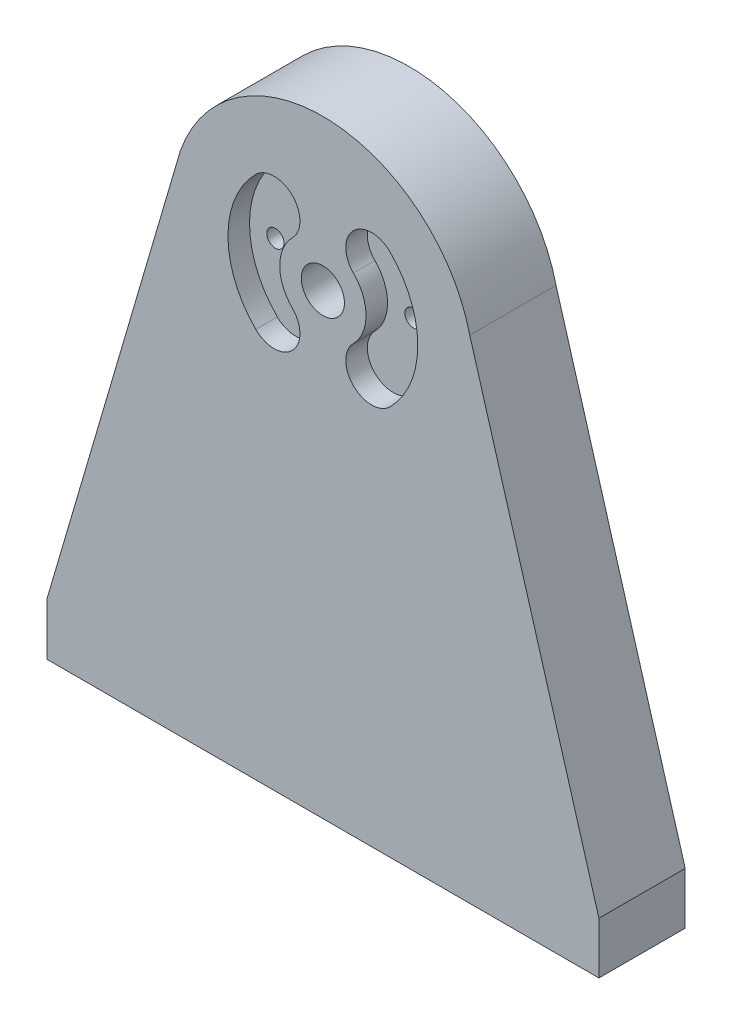
SolidWorks part; units mm, degrees
material "Plain Carbon Steel"
ref_plane "Front Plane" through (0, 0, 0) normal (0, 0, 1) x (1, 0, 0)
ref_plane "Top Plane" through (0, 0, 0) normal (0, 1, 0) x (1, 0, 0)
ref_plane "Right Plane" through (0, 0, 0) normal (1, 0, 0) x (0, 0, -1)
sketch "Post Plate Profile" plane through (0, 0, 0) normal (0, 0, 1) x (1, 0, 0)
  line L1 (-32, 0) -> (32, 0)
  line L2 (32, 0) -> (32, 6)
  line L3 (32, 6) -> (17.0272, 57.0405)
  line L4 (-32, 0) -> (-32, 6)
  line L5 (-32, 6) -> (-16.5115, 58.7982)
  arc A0 (17.0272, 57.0405) -> (-16.5115, 58.7982) centre (0, 53) ccw
  dimension "D1" = 17.5
  dimension "D2" = 32
  dimension "D3" = 6
  dimension "D4" = 53
  dimension "D5" = 32
  dimension "D6" = 64
  dimension "D7" = 51.0405
  dimension "D8" = 52.7982
  dimension "D9" = 17.476
extrude "Post Plate 10mm" add sketch "Post Plate Profile" along normal blind 10
sketch "Upper Slot Profile" plane through (0, 0, 0) normal (0, -1, 0) x (1, 0, 0)
  line L0 (-32, 10) -> (-32, 0) construction
  line L2 (32, 10) -> (32, 0) construction
  circle A0 centre (22, 5) radius 2.5
  circle A1 centre (-22, 5) radius 2.5
  dimension "D1" = 5
  dimension "D2" = 5
  dimension "D3" = 5
  dimension "D4" = 10
  dimension "D5" = 10
  dimension "D6" = 5
extrude "Upper Slot Cut" cut sketch "Upper Slot Profile" against normal blind 10
sketch "Upper Slot Relief Profile" plane through (0, 0, 0) normal (0, -1, 0) x (1, 0, 0)
  circle A0 centre (22, 5) radius 2.1
  circle A1 centre (-22, 5) radius 2.1
  dimension "D1" = 4.2
  dimension "D2" = 4.2
extrude "Upper Slot Relief Cut" cut sketch "Upper Slot Relief Profile" against normal blind 12.4
sketch "Long Slot Profile" plane through (0, 0, 0) normal (0, -1, 0) x (1, 0, 0)
  line L0 (-32, 10) -> (-32, 0) construction
  line L2 (-32, 0) -> (32, 0) construction
  circle A0 centre (-8, 5) radius 1
  circle A1 centre (8, 5) radius 1
  dimension "D1" = 2
  dimension "D5" = 2
  dimension "D2" = 8
  dimension "D3" = 24
  dimension "D4" = 5
  dimension "D6" = 5
extrude "Long Slot Cut 55 Deep" cut sketch "Long Slot Profile" against normal blind 55
sketch "Shaft Bore Ø5 Profile" plane through (0, 0, 10) normal (0, 0, 1) x (1, 0, 0)
  circle A0 centre (0, 53) radius 2.5
  dimension "D1" = 5
extrude "Shaft Bore Ø5" cut sketch "Shaft Bore Ø5 Profile" against normal blind 55
sketch "Pivot Recess Profile" plane through (0, 0, 10) normal (0, 0, 1) x (1, 0, 0)
  arc A0 (-3.5355, 56.5355) -> (-3.5355, 49.4645) centre (0, 53) ccw
  arc A1 (7.7782, 45.2218) -> (7.7782, 60.7782) centre (0, 53) ccw
  arc A2 (3.5355, 49.4645) -> (7.7782, 45.2218) centre (5.6569, 47.3431) ccw
  arc A3 (3.5355, 56.5355) -> (7.7782, 60.7782) centre (5.6569, 58.6569) cw
  arc A4 (-3.5355, 49.4645) -> (-7.7782, 45.2218) centre (-5.6569, 47.3431) cw
  arc A5 (-3.5355, 56.5355) -> (-7.7782, 60.7782) centre (-5.6569, 58.6569) ccw
  arc A6 (-7.7782, 60.7782) -> (-7.7782, 45.2218) centre (0, 53) ccw
  circle A7 centre (0, 53) radius 11 construction
  arc A8 (3.5355, 49.4645) -> (3.5355, 56.5355) centre (0, 53) ccw
  circle A9 centre (0, 53) radius 5 construction
  point P16 (11, 53)
  point P21 (4.7815, 54.4619)
  dimension "D1" = 6
  dimension "D2" = 3
  dimension "D3" = 3
  dimension "D4" = 3
  dimension "D5" = 11
  dimension "D11" = 3
  dimension "D6" = 5.6569
  dimension "D7" = 5.6569
  dimension "D8" = 5.6569
  dimension "D9" = 5.6569
  dimension "D10" = 5.6569
  dimension "D12" = 8
extrude "Pivot Recess 2.5 Deep" cut sketch "Pivot Recess Profile" against normal blind 2.5
sketch "Lower Slot Profile" plane through (0, 0, 7.5) normal (0, 0, 1) x (1, 0, 0)
  circle A0 centre (8, 53) radius 1
  circle A1 centre (-8, 53) radius 1
  circle A2 centre (0, 53) radius 2.5 construction
  arc A3 (3.5355, 49.4645) -> (7.7782, 45.2218) centre (5.6569, 47.3431) ccw construction
  dimension "D1" = 2
  dimension "D2" = 2
  dimension "D3" = 8
  dimension "D4" = 8
  dimension "D5" = 5.6569
extrude "Lower Slot Cut" cut sketch "Lower Slot Profile" against normal blind 5
